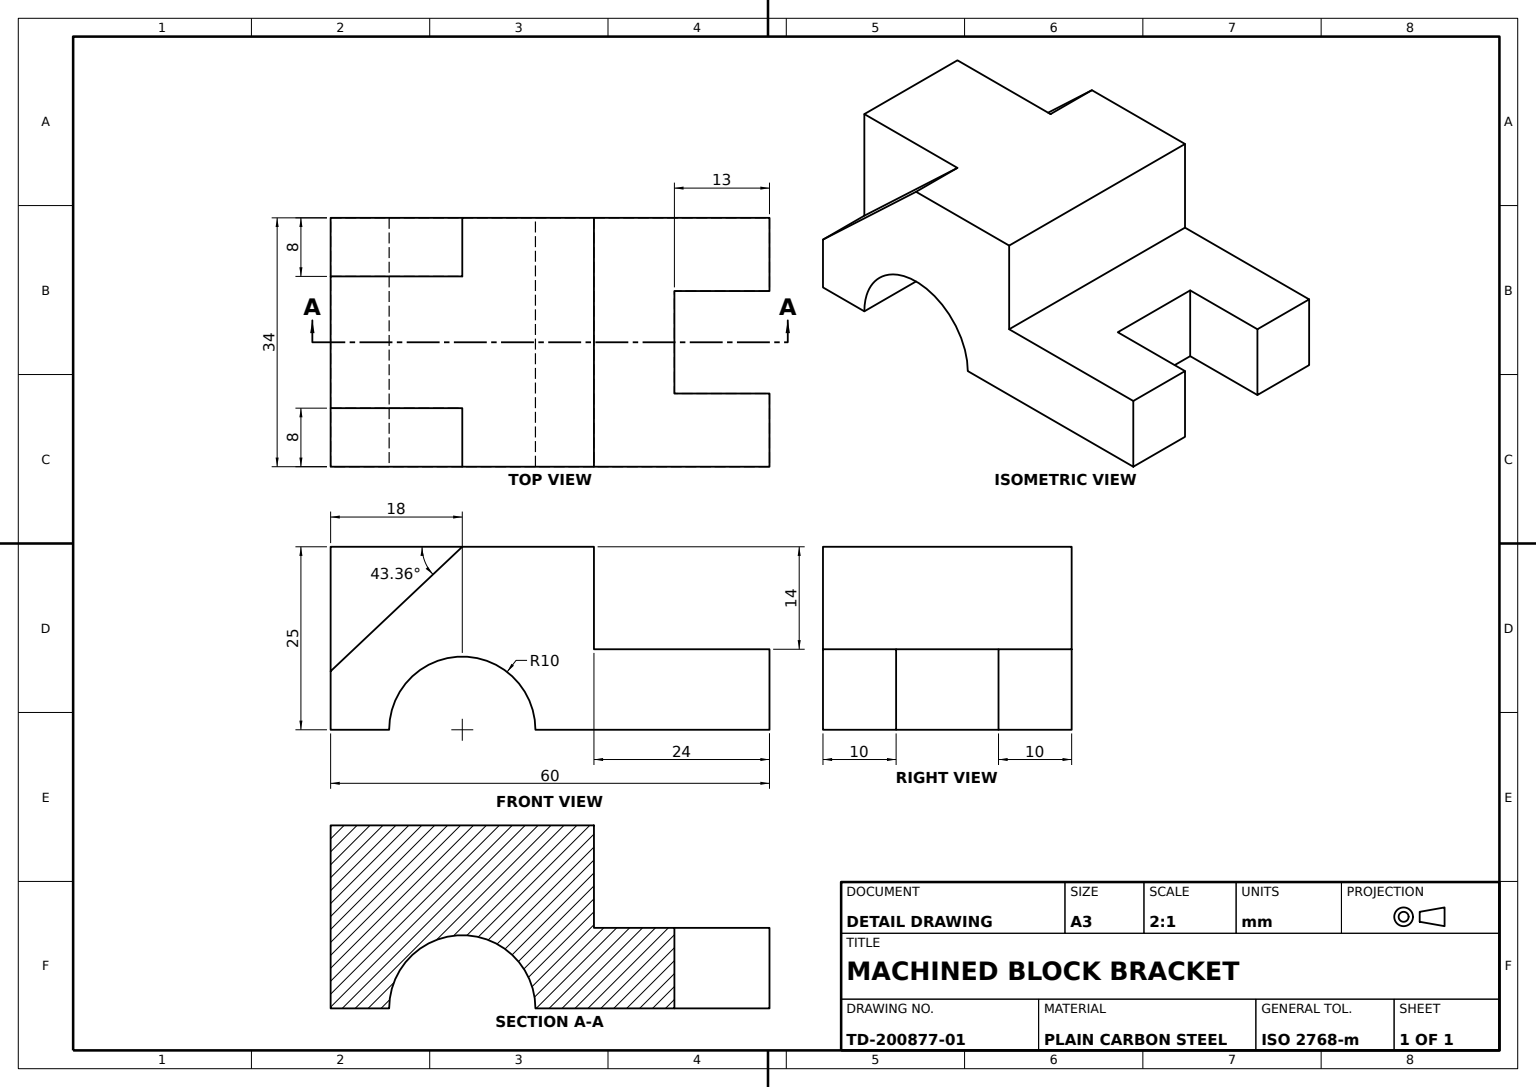
SolidWorks part; units mm, degrees
material "Plain Carbon Steel"
ref_plane "Front Plane" through (0, 0, 0) normal (0, 0, 1) x (1, 0, 0)
ref_plane "Top Plane" through (0, 0, 0) normal (0, 1, 0) x (1, 0, 0)
ref_plane "Right Plane" through (0, 0, 0) normal (1, 0, 0) x (0, 0, -1)
sketch "Block Profile Sketch" plane through (0, 0, 0) normal (1, 0, 0) x (0, 0, -1)
  line L1 (-30, 12.5) -> (30, 12.5)
  line L2 (-30, 12.5) -> (-30, -12.5)
  line L3 (-30, -12.5) -> (30, -12.5)
  line L4 (30, 12.5) -> (30, -12.5)
  line L5 (-30, 12.5) -> (30, -12.5) construction
  line L6 (-30, -12.5) -> (30, 12.5) construction
  point P0 (0, 0)
  dimension "D1" = 60
  dimension "D2" = 25
extrude "Base Block" add sketch "Block Profile Sketch" along normal blind 34
sketch "Step Cut Profile Sketch" plane through (34, 0, 0) normal (1, 0, 0) x (0, 0, -1)
  line L0 (30, -12.5) -> (30, 12.5) construction
  line L1 (30, 12.5) -> (6, 12.5)
  line L2 (30, 12.5) -> (30, -1.5)
  line L3 (30, -1.5) -> (6, -1.5)
  line L4 (6, 12.5) -> (6, -1.5)
  line L5 (-30, -12.5) -> (30, -12.5) construction
  line L6 (-22, -12.5) -> (-2, -12.5)
  arc A0 (-22, -12.5) -> (-2, -12.5) centre (-12, -12.5) cw
  dimension "D1" = 24
  dimension "D2" = 14
  dimension "D3" = 42
  dimension "D4" = 20
extrude "Stepped Through Cut" cut sketch "Step Cut Profile Sketch" against normal blind 34
sketch "Notch Profile Sketch" plane through (0, 12.5, 0) normal (0, 1, 0) x (1, 0, 0)
  line L5 (0, 30) -> (34, 30) construction
  line L6 (10, 30) -> (24, 30)
  line L7 (10, 30) -> (10, 17)
  line L8 (10, 17) -> (24, 17)
  line L9 (24, 30) -> (24, 17)
  dimension "D1" = 13
  dimension "D2" = 14
  dimension "D3" = 10
extrude "Side Notch Through Cut" cut sketch "Notch Profile Sketch" against normal blind 34
sketch "Slot Sketch" plane through (34, 0, 0) normal (1, 0, 0) x (0, 0, -1)
  line L0 (-30, -12.5) -> (-30, -4.5)
  line L1 (-30, 12.5) -> (-30, -12.5) construction
  line L2 (-30, -4.5) -> (-12, 12.5)
  line L3 (6, 12.5) -> (-30, 12.5) construction
  line L4 (-30, -4.5) -> (-30, 12.5)
  line L5 (-30, 12.5) -> (-12, 12.5)
  line M3 (6, 12.5) -> (-30, 12.5)
  line M4 (-30, 12.5) -> (-30, -12.5)
  dimension "D1" = 18
  dimension "D2" = 8
extrude "Slot 18x8 Depth 8" cut sketch "Slot Sketch" against normal blind 8 contours L2 M4 M3
sketch "Arch Relief Sketch" plane through (0, 0, 0) normal (-1, 0, 0) x (0, 0, 1)
  line L0 (30, -12.5) -> (30, -4.5)
  line L1 (30, 12.5) -> (30, -12.5) construction
  line L2 (30, -4.5) -> (12, 12.5)
  line L3 (-6, 12.5) -> (30, 12.5) construction
  line L4 (12, 12.5) -> (-6, 12.5)
  line L5 (12, 12.5) -> (30, 12.5)
  line L6 (30, 12.5) -> (30, -4.5)
  line M7 (30, -12.5) -> (30, 12.5)
  line M8 (30, 12.5) -> (-6, 12.5)
  dimension "D1" = 8
  dimension "D2" = 18
extrude "Arch Relief Cut" cut sketch "Arch Relief Sketch" against normal blind 8 contours L2 M7 M8
